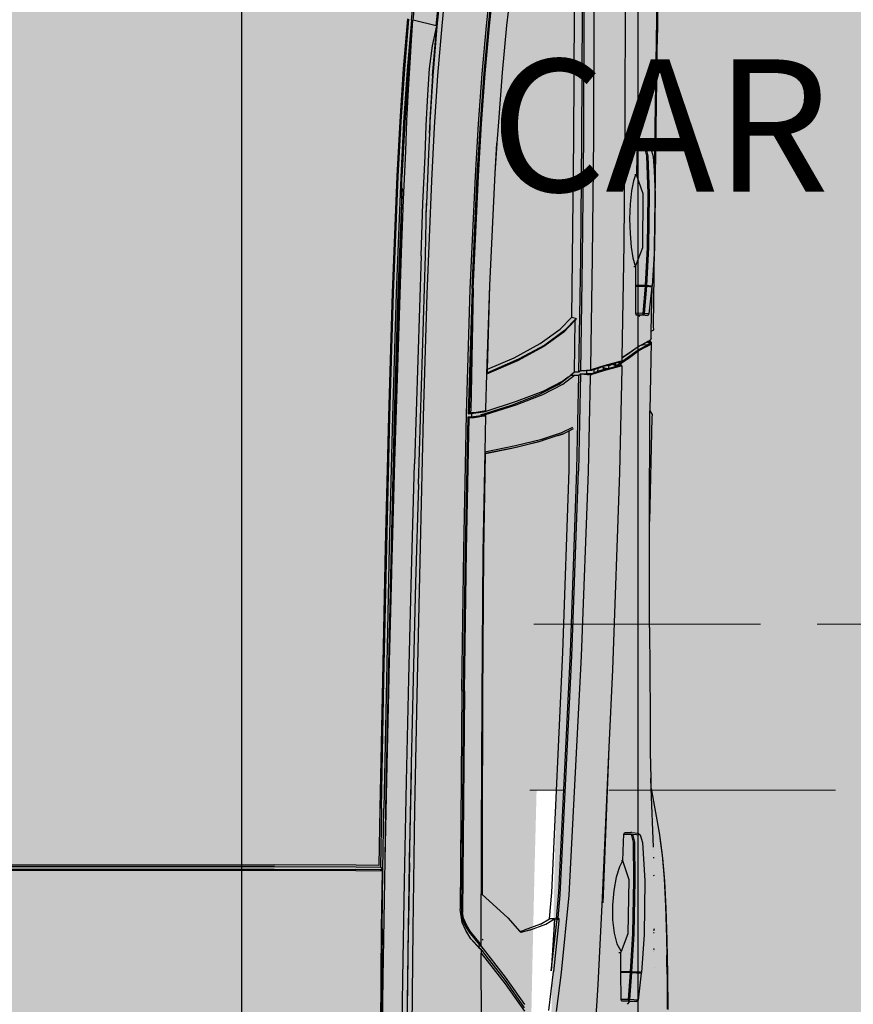
# Model space of a CAD drawing. Units: inches. Extents: x 1884 to 2398, y 474 to 1488.
# Tile 12 of 39: x 2231 to 2275, y 620 to 672. Entities that reach past the tile are written whole.
import ezdxf

# ---------------------------------------------------------------- set-up
doc = ezdxf.new("R2010")
doc.units = ezdxf.units.IN
doc.header["$MEASUREMENT"] = 0
doc.linetypes.add('ACAD_ISO02W100', pattern=[15, 12, -3])
doc.layers.get('0').update_dxf_attribs({"color": 250})
for name, color, linetype, lineweight in [('A-ANNO-DIMS', 2, 'Continuous', 18), ('A-FLOR-OVHD', 8, 'ACAD_ISO02W100', 18), ('C-VEHI', 8, 'Continuous', 18)]:
    doc.layers.add(name, color=color, linetype=linetype, lineweight=lineweight)
doc.layers.add('Edges', color=250, linetype='Continuous')
doc.layers.add('L-PVMT-PATT', color=9, linetype='Continuous', lineweight=13, true_color=0xc7c8ca)
doc.styles.get("Standard").update_dxf_attribs({"font": 'arial.ttf'})
doc.dimstyles.get("Standard").update_dxf_attribs({"dimtxt": 7, "dimasz": 0.18, "dimexe": 0.18, "dimexo": 0.0625, "dimgap": 0.09, "dimtad": 0, "dimtih": 1, "dimtoh": 1, "dimzin": 0, "dimdsep": 46, "dimlunit": 3, "dimtxsty": 'Standard', "dimcen": 0.09, "dimadec": 0, "dimazin": 0, "dimtfac": 1, "dimtofl": 0, "dimtmove": 0, "dimatfit": 3, "dimfxl": 1, "dimtolj": 1, "dimtzin": 0, "dimarcsym": 0})

# ---------------------------------------------------------------- blocks, each defined once
blk = doc.blocks.new('Nissan Qashqai pl')
at = {"layer": 'Edges'}
for p, q in [((10.4304, 12.8056), (10.4339, 12.8061)), ((10.4339, 12.8061), (10.4573, 12.8093)), ((10.4339, 12.8061), (10.4345, 12.8062)), ((10.4345, 12.8062), (10.4613, 12.8099)), ((10.4573, 12.8093), (10.4889, 12.8119)), ((10.4613, 12.8099), (10.4926, 12.8125)), ((10.4889, 12.8119), (10.526, 12.8138)), ((10.4926, 12.8125), (10.5294, 12.8143)), ((10.526, 12.8138), (10.569, 12.8151)), ((10.5294, 12.8143), (10.5719, 12.8156)), ((10.569, 12.8151), (10.5919, 12.8155)), ((10.5719, 12.8156), (10.6176, 12.8164)), ((10.5919, 12.8155), (10.6151, 12.8159)), ((10.5981, 12.8157), (10.5919, 12.8155)), ((10.6174, 12.816), (10.5981, 12.8157)), ((10.6151, 12.8159), (10.6644, 12.8162)), ((10.6176, 12.8164), (10.6651, 12.8167)), ((9.2517, 12.8031), (9.351, 12.803)), ((9.2517, 12.8031), (9.5372, 12.7983)), ((9.641, 12.7991), (9.351, 12.803)), ((9.5052, 12.7918), (9.5069, 12.7941)), ((9.5061, 12.7878), (9.5069, 12.7941)), ((9.5069, 12.7941), (9.5176, 12.7972)), ((9.5176, 12.7972), (9.5372, 12.7983)), ((9.5372, 12.7983), (9.5689, 12.7999)), ((9.5689, 12.7999), (9.641, 12.7991)), ((9.641, 12.7991), (9.6921, 12.7956)), ((9.7466, 12.7978), (9.641, 12.7991)), ((9.692, 12.7943), (9.6913, 12.7886)), ((9.6921, 12.7956), (9.692, 12.7943)), ((9.6922, 12.7943), (9.692, 12.7943)), ((9.6922, 12.7943), (9.6921, 12.7956)), ((9.7526, 12.7946), (9.6921, 12.7956)), ((9.6922, 12.7885), (9.693, 12.7955)), ((9.6922, 12.7885), (9.6922, 12.7943)), ((9.693, 12.7955), (9.7296, 12.7914)), ((9.7511, 12.7979), (9.7466, 12.7978)), ((9.7526, 12.7946), (9.7511, 12.7979)), ((9.7623, 12.7945), (9.7526, 12.7946)), ((9.7623, 12.7945), (9.7643, 12.7937)), ((9.7643, 12.7937), (9.7652, 12.7927)), ((9.7643, 12.7937), (9.7648, 12.7929)), ((9.7648, 12.7929), (9.7648, 12.7929)), ((9.7648, 12.7929), (9.7664, 12.7902)), ((9.7667, 12.7933), (9.7665, 12.7907)), ((9.7677, 12.7944), (9.7667, 12.7933)), ((9.7676, 12.7931), (9.7667, 12.7933)), ((9.7673, 12.7899), (9.7676, 12.7931)), ((9.769, 12.7926), (9.7676, 12.7931)), ((9.7677, 12.7944), (9.7677, 12.7944)), ((9.77, 12.7936), (9.7677, 12.7944)), ((9.7677, 12.7944), (9.8598, 12.7928)), ((9.7734, 12.7884), (9.77, 12.7936)), ((9.8598, 12.7928), (9.8614, 12.7937)), ((9.8614, 12.7937), (9.8647, 12.7956)), ((9.8647, 12.7956), (9.869, 12.7954)), ((9.869, 12.7954), (10.0085, 12.7922)), ((10.1513, 12.7924), (10.2677, 12.793)), ((10.2677, 12.793), (10.3189, 12.7931)), ((10.3189, 12.7931), (10.3537, 12.7939)), ((10.3537, 12.7939), (10.3832, 12.7945)), ((10.3679, 12.7944), (10.3537, 12.7939)), ((10.3679, 12.7944), (10.4275, 12.8051)), ((10.4468, 12.7976), (10.3679, 12.7944)), ((10.4275, 12.8051), (10.4304, 12.8056)), ((10.4503, 12.7976), (10.4502, 12.7976)), ((10.4603, 12.7976), (10.4613, 12.7978)), ((10.4838, 12.7977), (10.4852, 12.7982)), ((10.5565, 12.7985), (10.5591, 12.7977)), ((10.5615, 12.7978), (10.5617, 12.7985)), ((10.583, 12.7984), (10.5834, 12.798)), ((10.5836, 12.798), (10.5831, 12.7984)), ((10.5847, 12.798), (10.5841, 12.7984)), ((10.5873, 12.7981), (10.5873, 12.7981)), ((10.6087, 12.7983), (10.6087, 12.7984)), ((9.5037, 12.7806), (9.5045, 12.7814)), ((9.5052, 12.7918), (9.5044, 12.7856)), ((9.5044, 12.7856), (9.5045, 12.7814)), ((9.5045, 12.7814), (9.5045, 12.7759)), ((9.5168, 12.7904), (9.5061, 12.7878)), ((9.5061, 12.7856), (9.5167, 12.7883)), ((9.5063, 12.7755), (9.5061, 12.7856)), ((9.5167, 12.7883), (9.5679, 12.7899)), ((9.5679, 12.792), (9.5168, 12.7904)), ((9.5678, 12.7837), (9.5426, 12.7747)), ((9.64, 12.7831), (9.5678, 12.7837)), ((9.6401, 12.7914), (9.5679, 12.792)), ((9.5679, 12.7899), (9.64, 12.7892)), ((9.64, 12.7892), (9.6912, 12.7865)), ((9.6645, 12.7737), (9.64, 12.7831)), ((9.6913, 12.7886), (9.6401, 12.7914)), ((9.6912, 12.7811), (9.6911, 12.7796)), ((9.6911, 12.7796), (9.6911, 12.7732)), ((9.6913, 12.7886), (9.6912, 12.7865)), ((9.6912, 12.7865), (9.6912, 12.7811)), ((9.692, 12.7811), (9.6912, 12.7811)), ((9.692, 12.7811), (9.6921, 12.7864)), ((9.692, 12.7796), (9.692, 12.7811)), ((9.692, 12.7733), (9.692, 12.7796)), ((9.6922, 12.7885), (9.6921, 12.7864)), ((9.6921, 12.7864), (9.7288, 12.7832)), ((9.7288, 12.7854), (9.6922, 12.7885)), ((9.7288, 12.7832), (9.7287, 12.7734)), ((9.7296, 12.7914), (9.7288, 12.7854)), ((9.7306, 12.7834), (9.7288, 12.7854)), ((9.7288, 12.7854), (9.7288, 12.7832)), ((9.7288, 12.7832), (9.7306, 12.7834)), ((9.7296, 12.7914), (9.7314, 12.7895)), ((9.7305, 12.7738), (9.7306, 12.7834)), ((9.7305, 12.7738), (9.7313, 12.7798)), ((9.7306, 12.7834), (9.7314, 12.7895)), ((9.7314, 12.7895), (9.7313, 12.7798)), ((9.733, 12.7782), (9.7313, 12.7798)), ((9.7652, 12.7927), (9.7665, 12.7907)), ((9.7665, 12.7904), (9.7664, 12.7902)), ((9.7664, 12.7902), (9.7674, 12.7885)), ((9.7665, 12.7907), (9.7676, 12.7889)), ((9.7673, 12.7897), (9.7673, 12.7899)), ((9.7673, 12.7897), (9.7676, 12.7889)), ((9.7674, 12.7885), (9.7728, 12.7781)), ((9.7676, 12.7889), (9.7684, 12.7875)), ((9.7676, 12.7887), (9.7678, 12.7882)), ((9.7684, 12.7875), (9.7717, 12.781)), ((9.7712, 12.7892), (9.769, 12.7926)), ((9.7707, 12.7848), (9.7709, 12.7893)), ((9.7717, 12.781), (9.7707, 12.7848)), ((9.7709, 12.7893), (9.7712, 12.7892)), ((9.7724, 12.7874), (9.7712, 12.7892)), ((9.7717, 12.781), (9.7738, 12.7771)), ((9.7778, 12.777), (9.7724, 12.7874)), ((9.7788, 12.778), (9.7734, 12.7884)), ((9.8643, 12.7927), (9.8598, 12.7928)), ((10.0085, 12.7922), (9.8643, 12.7927)), ((10.0124, 12.7922), (10.0085, 12.7922)), ((10.1513, 12.7924), (10.0124, 12.7922)), ((10.4282, 12.7775), (10.4299, 12.7798)), ((10.4291, 12.77), (10.4299, 12.7798)), ((10.4299, 12.7798), (10.4406, 12.7829)), ((10.4406, 12.7829), (10.4919, 12.7858)), ((10.4919, 12.7858), (10.564, 12.7851)), ((10.564, 12.7851), (10.6151, 12.7813)), ((10.615, 12.7803), (10.6142, 12.7686)), ((10.6151, 12.7813), (10.615, 12.7803)), ((10.615, 12.7676), (10.6151, 12.7803)), ((10.6151, 12.7803), (10.615, 12.7803)), ((10.6151, 12.7803), (10.6151, 12.7813)), ((10.6151, 12.7685), (10.616, 12.7812)), ((10.616, 12.7812), (10.6526, 12.7768)), ((9.5045, 12.7759), (9.5063, 12.7755)), ((9.5063, 12.7755), (9.5168, 12.7751)), ((9.5168, 12.7751), (9.5423, 12.7746)), ((9.5423, 12.7746), (9.5422, 12.7736)), ((9.5422, 12.7736), (9.5422, 12.7725)), ((9.5422, 12.7736), (9.5424, 12.7735)), ((9.5426, 12.7747), (9.5423, 12.7746)), ((9.5426, 12.7747), (9.5424, 12.7735)), ((9.5424, 12.7735), (9.5503, 12.7706)), ((9.5503, 12.7706), (9.5641, 12.7681)), ((9.5641, 12.7681), (9.5818, 12.766)), ((9.6215, 12.766), (9.6395, 12.7676)), ((9.6395, 12.7676), (9.654, 12.7697)), ((9.654, 12.7697), (9.6633, 12.7726)), ((9.6633, 12.7726), (9.6645, 12.7737)), ((9.6655, 12.7733), (9.6645, 12.7737)), ((9.6655, 12.7733), (9.6911, 12.7732)), ((9.6655, 12.7713), (9.6655, 12.7733)), ((9.6911, 12.7732), (9.692, 12.7733)), ((9.692, 12.7733), (9.7287, 12.7734)), ((9.7287, 12.7734), (9.7305, 12.7738)), ((9.7728, 12.7781), (9.7832, 12.7637)), ((9.7738, 12.7771), (9.7842, 12.7627)), ((9.7883, 12.7626), (9.7778, 12.777)), ((9.7894, 12.7636), (9.7788, 12.778)), ((10.4263, 12.7665), (10.4274, 12.7674)), ((10.4282, 12.7775), (10.4274, 12.7679)), ((10.4274, 12.7679), (10.4274, 12.7674)), ((10.4274, 12.7674), (10.4275, 12.7586)), ((10.4398, 12.7724), (10.4291, 12.77)), ((10.4291, 12.7677), (10.4398, 12.7701)), ((10.4293, 12.7579), (10.4291, 12.7677)), ((10.4909, 12.773), (10.4398, 12.7724)), ((10.4398, 12.7701), (10.4909, 12.7708)), ((10.5631, 12.7715), (10.4909, 12.773)), ((10.4909, 12.7708), (10.563, 12.7692)), ((10.563, 12.7692), (10.6142, 12.7663)), ((10.6142, 12.7686), (10.5631, 12.7715)), ((10.6142, 12.7686), (10.6142, 12.7677)), ((10.6142, 12.7677), (10.615, 12.7676)), ((10.6142, 12.7677), (10.6142, 12.7663)), ((10.6151, 12.7676), (10.615, 12.7676)), ((10.6518, 12.7657), (10.6151, 12.7685)), ((10.6151, 12.7676), (10.6151, 12.7685)), ((10.6151, 12.7662), (10.6151, 12.7676)), ((10.6526, 12.7768), (10.6518, 12.7657)), ((10.6526, 12.7768), (10.6543, 12.7749)), ((10.6537, 12.7658), (10.6543, 12.7749)), ((10.6543, 12.7749), (10.6543, 12.7656)), ((9.2886, 12.7594), (9.4673, 12.7589)), ((9.4673, 12.7589), (9.6358, 12.7575)), ((9.5818, 12.766), (9.6016, 12.7651)), ((9.6016, 12.7651), (9.6215, 12.766)), ((9.6358, 12.7575), (9.7887, 12.7552)), ((9.7832, 12.7637), (9.7887, 12.7552)), ((9.7842, 12.7627), (9.7891, 12.7552)), ((9.7933, 12.7549), (9.7883, 12.7626)), ((9.7887, 12.7552), (9.7891, 12.7552)), ((9.7891, 12.7552), (9.79, 12.7552)), ((9.7965, 12.7526), (9.7894, 12.7636)), ((9.79, 12.7552), (9.7931, 12.7552)), ((9.7931, 12.7552), (9.7934, 12.7535)), ((9.7931, 12.7552), (9.7933, 12.7549)), ((9.7933, 12.7549), (9.7941, 12.7541)), ((9.7934, 12.7535), (9.7938, 12.7538)), ((9.7934, 12.7535), (9.7937, 12.7524)), ((9.7941, 12.7541), (9.7943, 12.7535)), ((9.7955, 12.7516), (9.7943, 12.7535)), ((9.7943, 12.7535), (9.7964, 12.7453)), ((9.7983, 12.7541), (9.7965, 12.7526)), ((9.7977, 12.7535), (9.7967, 12.7526)), ((9.7982, 12.754), (9.7977, 12.7535)), ((9.7983, 12.7541), (9.7982, 12.754)), ((9.7986, 12.7526), (9.7982, 12.754)), ((9.7986, 12.7544), (9.7983, 12.7541)), ((9.7993, 12.755), (9.7986, 12.7544)), ((9.7999, 12.7522), (9.7993, 12.755)), ((9.7993, 12.755), (9.8024, 12.7549)), ((9.8024, 12.7549), (9.9426, 12.7518)), ((10.4293, 12.7579), (10.4275, 12.7586)), ((10.4398, 12.7573), (10.4293, 12.7579)), ((10.4653, 12.7564), (10.4398, 12.7573)), ((10.4653, 12.7561), (10.4652, 12.7545)), ((10.4908, 12.7648), (10.4653, 12.7564)), ((10.4653, 12.7564), (10.4653, 12.7561)), ((10.4653, 12.7564), (10.4653, 12.7564)), ((10.4653, 12.7564), (10.4653, 12.7561)), ((10.4653, 12.7561), (10.4653, 12.7561)), ((10.4653, 12.7561), (10.4732, 12.7517)), ((10.563, 12.7633), (10.4908, 12.7648)), ((10.5867, 12.7545), (10.563, 12.7633)), ((10.5769, 12.7484), (10.5863, 12.7537)), ((10.5863, 12.7537), (10.5867, 12.7545)), ((10.5885, 12.7538), (10.5867, 12.7545)), ((10.5885, 12.751), (10.5885, 12.7538)), ((10.6141, 12.7537), (10.5885, 12.7538)), ((10.6142, 12.766), (10.6141, 12.7537)), ((10.6141, 12.7537), (10.615, 12.7537)), ((10.6142, 12.7663), (10.6142, 12.766)), ((10.615, 12.7537), (10.6151, 12.7659)), ((10.6517, 12.754), (10.615, 12.7537)), ((10.6151, 12.7662), (10.6518, 12.7634)), ((10.6151, 12.7659), (10.6151, 12.7662)), ((10.6518, 12.7634), (10.6517, 12.754)), ((10.6535, 12.7546), (10.6517, 12.754)), ((10.6536, 12.7639), (10.6518, 12.7657)), ((10.6518, 12.7657), (10.6518, 12.7634)), ((10.6518, 12.7634), (10.6536, 12.7639)), ((10.6543, 12.7656), (10.6535, 12.7546)), ((10.6535, 12.7546), (10.6536, 12.7639)), ((10.6536, 12.7639), (10.6537, 12.7658)), ((10.6537, 12.7658), (10.6543, 12.7656)), ((10.6578, 12.7628), (10.6543, 12.7656)), ((9.7937, 12.7524), (9.7992, 12.7308)), ((9.7963, 12.7523), (9.7955, 12.7516)), ((9.7963, 12.7523), (9.7963, 12.7524)), ((9.7964, 12.7524), (9.7963, 12.7523)), ((9.7992, 12.7476), (9.7963, 12.7523)), ((9.7967, 12.7526), (9.7964, 12.7524)), ((9.7964, 12.7525), (9.7964, 12.7524)), ((9.7964, 12.7524), (9.7996, 12.7475)), ((9.7964, 12.7453), (9.7992, 12.7476)), ((9.7964, 12.7453), (9.7973, 12.7418)), ((9.7965, 12.7526), (9.7967, 12.7526)), ((9.7967, 12.7526), (9.7986, 12.7526)), ((9.7977, 12.7431), (9.7973, 12.7418)), ((9.7973, 12.7418), (9.7977, 12.7409)), ((9.7973, 12.7418), (9.7977, 12.7399)), ((9.7977, 12.7444), (9.7985, 12.7451)), ((9.7985, 12.7451), (9.7977, 12.7431)), ((9.7977, 12.7431), (9.7977, 12.7444)), ((9.7977, 12.7399), (9.7977, 12.7409)), ((9.7977, 12.7409), (9.7987, 12.7388)), ((9.7977, 12.7399), (9.7978, 12.7397)), ((9.7989, 12.7461), (9.7985, 12.7451)), ((9.7988, 12.7516), (9.7986, 12.7526)), ((9.7998, 12.7477), (9.7988, 12.7516)), ((9.7998, 12.7466), (9.7989, 12.7461)), ((9.7998, 12.7466), (9.7992, 12.7476)), ((9.7996, 12.7475), (9.7998, 12.7477)), ((9.8002, 12.7461), (9.7996, 12.7475)), ((9.8001, 12.7468), (9.7996, 12.7475)), ((9.8001, 12.7468), (9.7998, 12.7477)), ((9.8003, 12.7458), (9.7998, 12.7466)), ((9.8054, 12.7307), (9.7999, 12.7522)), ((9.8002, 12.7461), (9.8001, 12.7468)), ((9.8003, 12.7458), (9.8002, 12.7461)), ((9.8027, 12.7364), (9.8003, 12.7458)), ((9.9426, 12.7518), (10.2081, 12.7424)), ((10.2081, 12.7424), (10.312, 12.7377)), ((10.4732, 12.7517), (10.4871, 12.7474)), ((10.4871, 12.7474), (10.5048, 12.744)), ((10.5048, 12.744), (10.5246, 12.7423)), ((10.5246, 12.7423), (10.5445, 12.7425)), ((10.5445, 12.7425), (10.5625, 12.7446)), ((10.5625, 12.7446), (10.5769, 12.7484)), ((9.7987, 12.7388), (9.7978, 12.7397)), ((9.7978, 12.7397), (9.7987, 12.7362)), ((9.7987, 12.7388), (9.7992, 12.7377)), ((9.7987, 12.7362), (9.7992, 12.7377)), ((9.7987, 12.7362), (9.8002, 12.7301)), ((9.7992, 12.7377), (9.8027, 12.7364)), ((9.7992, 12.7308), (9.8044, 12.7151)), ((9.8002, 12.7301), (9.8008, 12.7285)), ((9.8008, 12.7285), (9.8014, 12.7303)), ((9.8008, 12.7285), (9.8014, 12.7265)), ((9.8014, 12.7303), (9.8031, 12.7349)), ((9.8043, 12.7303), (9.8014, 12.7303)), ((9.8031, 12.7349), (9.8027, 12.7364)), ((9.8043, 12.7303), (9.8031, 12.7349)), ((9.8044, 12.73), (9.8043, 12.7303)), ((9.8067, 12.7229), (9.8044, 12.73)), ((9.8106, 12.715), (9.8054, 12.7307)), ((10.312, 12.7377), (10.5214, 12.7293)), ((10.312, 12.7377), (10.5147, 12.7285)), ((10.5147, 12.7285), (10.6318, 12.7228)), ((9.4919, 12.7173), (9.3194, 12.7179)), ((9.6538, 12.7157), (9.4919, 12.7173)), ((9.802, 12.7133), (9.6538, 12.7157)), ((9.8014, 12.7265), (9.803, 12.723)), ((9.8014, 12.7265), (9.8026, 12.723)), ((9.803, 12.723), (9.8026, 12.723)), ((9.8026, 12.723), (9.8046, 12.7171)), ((9.8067, 12.7229), (9.803, 12.723)), ((9.8044, 12.7151), (9.8051, 12.7132)), ((9.8046, 12.7171), (9.8086, 12.7171)), ((9.8046, 12.7171), (9.8055, 12.7143)), ((9.8055, 12.7143), (9.8058, 12.7073)), ((9.8086, 12.7171), (9.8067, 12.7229)), ((9.8096, 12.7142), (9.8086, 12.7171)), ((9.8098, 12.7073), (9.8096, 12.7142)), ((9.8112, 12.7131), (9.8106, 12.715)), ((10.6318, 12.7228), (10.6955, 12.7184)), ((9.3198, 12.7039), (9.4922, 12.7033)), ((9.4936, 12.7013), (9.3225, 12.7021)), ((9.4922, 12.7033), (9.654, 12.7018)), ((9.6552, 12.6997), (9.4936, 12.7013)), ((9.654, 12.7018), (9.8061, 12.6994)), ((9.8051, 12.7132), (9.802, 12.7133)), ((9.8061, 12.6994), (9.8051, 12.7132)), ((9.8058, 12.7073), (9.8098, 12.7073)), ((9.8058, 12.7073), (9.8061, 12.6994)), ((9.8101, 12.6993), (9.8098, 12.7073)), ((9.8101, 12.6993), (9.8112, 12.7131)), ((9.8143, 12.713), (9.8112, 12.7131)), ((9.9414, 12.71), (9.8143, 12.713)), ((10.19, 12.7008), (9.9414, 12.71)), ((10.5113, 12.6839), (10.19, 12.7008)), ((9.4936, 12.6904), (9.3225, 12.6911)), ((9.6552, 12.6888), (9.4936, 12.6904)), ((9.8078, 12.6971), (9.6552, 12.6997)), ((9.7337, 12.6875), (9.6552, 12.6888)), ((9.7337, 12.6875), (9.7357, 12.6935)), ((9.7499, 12.6721), (9.7337, 12.6875)), ((9.7357, 12.6935), (9.7378, 12.6924)), ((9.7357, 12.6935), (9.7519, 12.678)), ((9.7378, 12.6924), (9.754, 12.677)), ((9.8078, 12.6913), (9.7378, 12.6924)), ((9.8061, 12.6994), (9.8078, 12.6971)), ((9.8078, 12.6971), (9.8078, 12.6913)), ((9.8078, 12.6913), (9.8119, 12.6862)), ((9.8119, 12.697), (9.8101, 12.6993)), ((9.8101, 12.6993), (9.9411, 12.6966)), ((9.9393, 12.6944), (9.8119, 12.697)), ((9.8119, 12.6912), (9.8119, 12.697)), ((9.8241, 12.6756), (9.8119, 12.6912)), ((9.8119, 12.6862), (9.8119, 12.6912)), ((9.8891, 12.6741), (9.8818, 12.6891)), ((9.8867, 12.6842), (9.8838, 12.6901)), ((10.1849, 12.6857), (9.9393, 12.6944)), ((10.1894, 12.6879), (9.9411, 12.6966)), ((10.5109, 12.6721), (10.1894, 12.6879)), ((9.7519, 12.678), (9.7713, 12.6512)), ((9.754, 12.677), (9.7733, 12.6502)), ((9.8147, 12.6826), (9.8119, 12.6862)), ((9.8147, 12.6826), (9.8147, 12.6826)), ((9.8147, 12.6826), (9.8201, 12.6756)), ((9.8241, 12.6706), (9.8147, 12.6826)), ((9.8201, 12.6756), (9.8338, 12.6486)), ((9.8378, 12.6485), (9.8241, 12.6756)), ((9.9393, 12.684), (9.8867, 12.6842)), ((9.8911, 12.675), (9.8867, 12.6842)), ((9.8978, 12.6472), (9.8891, 12.6741)), ((9.8911, 12.6749), (9.8911, 12.675)), ((9.8931, 12.6691), (9.8911, 12.6749)), ((9.8911, 12.6749), (9.8998, 12.6481)), ((10.1849, 12.6754), (9.9393, 12.684)), ((10.5079, 12.6703), (10.1849, 12.6857)), ((10.5079, 12.6607), (10.1849, 12.6754)), ((10.6152, 12.674), (10.5113, 12.6839)), ((10.6678, 12.6672), (10.6152, 12.674)), ((9.7692, 12.6453), (9.7499, 12.6721)), ((9.8378, 12.6435), (9.8241, 12.6706)), ((9.8931, 12.669), (9.8931, 12.6691)), ((9.8931, 12.669), (9.9018, 12.6421)), ((10.543, 12.6671), (10.5079, 12.6703)), ((10.543, 12.6576), (10.5079, 12.6607)), ((10.5417, 12.6693), (10.5109, 12.6721)), ((10.5417, 12.6693), (10.5427, 12.6702)), ((10.5417, 12.6693), (10.543, 12.6671)), ((10.5436, 12.6687), (10.5427, 12.6702)), ((10.5427, 12.6702), (10.5458, 12.67)), ((10.544, 12.6678), (10.543, 12.6671)), ((10.543, 12.6646), (10.543, 12.6671)), ((10.543, 12.6646), (10.543, 12.6576)), ((10.5439, 12.6646), (10.543, 12.6646)), ((10.5502, 12.6526), (10.543, 12.6646)), ((10.544, 12.6678), (10.5436, 12.6687)), ((10.5439, 12.6646), (10.613, 12.6601)), ((10.547, 12.6674), (10.544, 12.6678)), ((10.5458, 12.67), (10.6144, 12.6629)), ((10.613, 12.6601), (10.547, 12.6674)), ((10.6664, 12.6566), (10.6144, 12.6629)), ((9.7713, 12.6512), (9.7905, 12.6158)), ((9.7733, 12.6502), (9.7925, 12.6148)), ((9.8338, 12.6486), (9.8475, 12.613)), ((9.8516, 12.6129), (9.8378, 12.6485)), ((9.9066, 12.6119), (9.8978, 12.6472)), ((9.9086, 12.6129), (9.8998, 12.6481)), ((10.5502, 12.6456), (10.543, 12.6576)), ((10.5584, 12.6306), (10.5502, 12.6526)), ((9.7885, 12.6099), (9.7692, 12.6453)), ((9.8516, 12.6079), (9.8378, 12.6435)), ((9.9018, 12.6421), (9.9106, 12.6068)), ((10.5502, 12.6456), (10.5584, 12.6236)), ((10.5584, 12.6306), (10.5617, 12.619)), ((10.56, 12.6176), (10.5584, 12.6236)), ((10.6583, 12.6245), (10.6215, 12.5986)), ((10.6627, 12.6241), (10.6261, 12.5984)), ((10.6306, 12.5982), (10.6671, 12.6238)), ((9.8039, 12.5741), (9.7885, 12.6099)), ((9.7905, 12.6158), (9.8087, 12.574)), ((9.7925, 12.6148), (9.8107, 12.573)), ((9.8475, 12.613), (9.8611, 12.5708)), ((9.8652, 12.5704), (9.8516, 12.6129)), ((9.8652, 12.5654), (9.8516, 12.6079)), ((9.9149, 12.5705), (9.9066, 12.6119)), ((9.9169, 12.5714), (9.9086, 12.6129)), ((10.5419, 12.6018), (10.56, 12.6176)), ((10.56, 12.6176), (10.5617, 12.619)), ((9.2814, 12.6065), (9.3416, 12.5999)), ((9.3416, 12.5999), (9.4048, 12.5941)), ((9.9106, 12.6068), (9.9177, 12.5714)), ((10.51, 12.5666), (10.5419, 12.6018)), ((10.6215, 12.5986), (10.5796, 12.5655)), ((10.5892, 12.5659), (10.6306, 12.5982)), ((10.6261, 12.5984), (10.593, 12.5726)), ((9.3418, 12.5771), (9.2803, 12.5836)), ((9.3419, 12.5756), (9.2804, 12.5821)), ((9.4048, 12.5941), (9.471, 12.5888)), ((9.471, 12.5888), (9.4997, 12.5869)), ((9.5404, 12.5844), (9.4997, 12.5869)), ((9.4997, 12.5869), (9.5403, 12.5842)), ((9.5403, 12.5842), (9.6913, 12.5767)), ((9.6912, 12.5774), (9.5404, 12.5844)), ((9.3418, 12.5729), (9.2801, 12.5794)), ((9.4062, 12.5713), (9.3418, 12.5771)), ((9.4064, 12.5671), (9.3418, 12.5729)), ((9.4063, 12.5699), (9.3419, 12.5756)), ((9.4735, 12.5663), (9.4062, 12.5713)), ((9.4736, 12.5648), (9.4063, 12.5699)), ((9.8039, 12.5741), (9.6912, 12.5774)), ((9.6913, 12.5767), (9.8099, 12.573)), ((9.8087, 12.574), (9.8039, 12.5741)), ((9.8099, 12.573), (9.8087, 12.574)), ((9.8099, 12.573), (9.8107, 12.573)), ((9.8107, 12.573), (9.8573, 12.5716)), ((9.8573, 12.5716), (9.8603, 12.5715)), ((9.8603, 12.5715), (9.8605, 12.5696)), ((9.8611, 12.5708), (9.8603, 12.5715)), ((9.8605, 12.5696), (9.8626, 12.5564)), ((9.8612, 12.5707), (9.8611, 12.5708)), ((9.8612, 12.5707), (9.8615, 12.5688)), ((9.8615, 12.5688), (9.8635, 12.5556)), ((9.8652, 12.5706), (9.8664, 12.5714)), ((9.8652, 12.5706), (9.8665, 12.5695)), ((9.8652, 12.5704), (9.8652, 12.5706)), ((9.8652, 12.5704), (9.8652, 12.5704)), ((9.8652, 12.5704), (9.8652, 12.5654)), ((9.8655, 12.5687), (9.8652, 12.5704)), ((9.8675, 12.5555), (9.8655, 12.5687)), ((9.8665, 12.5695), (9.8664, 12.5714)), ((9.8664, 12.5714), (9.9149, 12.5705)), ((9.8686, 12.5562), (9.8665, 12.5695)), ((9.9149, 12.5705), (10.0505, 12.5681)), ((9.9177, 12.5714), (9.9169, 12.5714)), ((10.0501, 12.5695), (9.9177, 12.5714)), ((10.2453, 12.568), (10.0501, 12.5695)), ((10.0505, 12.5681), (10.2453, 12.5664)), ((10.4292, 12.5674), (10.2453, 12.568)), ((10.5719, 12.5682), (10.5709, 12.5675)), ((10.593, 12.5726), (10.584, 12.5655)), ((9.4739, 12.5621), (9.4064, 12.5671)), ((9.5437, 12.5619), (9.4735, 12.5663)), ((9.5438, 12.5605), (9.4736, 12.5648)), ((9.5443, 12.5579), (9.4739, 12.5621)), ((9.6953, 12.5549), (9.5437, 12.5619)), ((9.6954, 12.5535), (9.5438, 12.5605)), ((9.696, 12.551), (9.5443, 12.5579)), ((9.6953, 12.5549), (9.8598, 12.5517)), ((9.6953, 12.5549), (9.863, 12.5497)), ((9.8626, 12.5564), (9.8627, 12.5532)), ((9.8635, 12.5556), (9.8637, 12.5532)), ((9.8677, 12.5531), (9.8675, 12.5555)), ((9.8689, 12.5515), (9.8686, 12.5562)), ((10.2453, 12.5664), (10.4289, 12.5658)), ((10.4289, 12.5658), (10.5092, 12.5658)), ((10.5099, 12.5674), (10.4292, 12.5674)), ((10.5099, 12.5674), (10.5092, 12.5658)), ((10.5092, 12.5658), (10.5094, 12.5658)), ((10.5094, 12.5658), (10.51, 12.5666)), ((10.5783, 12.5659), (10.5094, 12.5658)), ((10.51, 12.5666), (10.5099, 12.5674)), ((10.5764, 12.5642), (10.5598, 12.5507)), ((10.5776, 12.5633), (10.5612, 12.5498)), ((10.5834, 12.5641), (10.57, 12.5517)), ((10.57, 12.5517), (10.5821, 12.5633)), ((10.5709, 12.5675), (10.5705, 12.5671)), ((10.5783, 12.5659), (10.5764, 12.5642)), ((10.5776, 12.5633), (10.5783, 12.5659)), ((10.5796, 12.5655), (10.5776, 12.5633)), ((10.5796, 12.5655), (10.5783, 12.5659)), ((10.5796, 12.562), (10.5796, 12.5655)), ((10.5838, 12.5653), (10.5821, 12.5633)), ((10.584, 12.5647), (10.5834, 12.5641)), ((10.584, 12.5655), (10.5838, 12.5653)), ((10.584, 12.5655), (10.5841, 12.5655)), ((10.584, 12.5654), (10.584, 12.5655)), ((10.5847, 12.5655), (10.584, 12.5647)), ((10.584, 12.5647), (10.584, 12.5654)), ((10.5851, 12.5659), (10.5841, 12.5655)), ((10.5841, 12.5655), (10.5847, 12.5655)), ((10.5851, 12.5659), (10.5847, 12.5655)), ((10.5851, 12.5659), (10.5892, 12.5659)), ((10.6988, 12.5662), (10.5892, 12.5659)), ((9.6954, 12.5535), (9.8641, 12.5483)), ((9.8644, 12.5459), (9.696, 12.551)), ((9.8629, 12.5516), (9.8598, 12.5517)), ((9.8637, 12.5532), (9.8627, 12.5532)), ((9.8627, 12.5532), (9.8629, 12.5516)), ((9.8629, 12.5516), (9.863, 12.5497)), ((9.8641, 12.5483), (9.863, 12.5497)), ((9.8643, 12.5532), (9.8637, 12.5532)), ((9.8637, 12.5532), (9.8638, 12.5508)), ((9.8638, 12.5508), (9.8641, 12.5483)), ((9.8677, 12.5531), (9.8643, 12.5532)), ((10.0472, 12.5423), (9.8644, 12.5459)), ((9.8678, 12.5507), (9.8677, 12.5531)), ((9.8681, 12.5482), (9.8678, 12.5507)), ((9.8681, 12.5482), (9.869, 12.5496)), ((10.0476, 12.5445), (9.8681, 12.5482)), ((9.869, 12.5496), (9.8689, 12.5515)), ((10.0477, 12.5459), (9.869, 12.5496)), ((10.2357, 12.5398), (10.0472, 12.5423)), ((10.2367, 12.5419), (10.0476, 12.5445)), ((10.2369, 12.5433), (10.0477, 12.5459)), ((10.2367, 12.5419), (10.5351, 12.5392)), ((10.2369, 12.5433), (10.5348, 12.5406)), ((10.5422, 12.542), (10.5348, 12.5406)), ((10.5522, 12.5465), (10.5422, 12.542)), ((10.5495, 12.5438), (10.5424, 12.5406)), ((10.5463, 12.541), (10.5551, 12.5457)), ((10.5589, 12.5451), (10.5479, 12.54)), ((10.5546, 12.546), (10.5495, 12.5438)), ((10.5598, 12.5507), (10.5522, 12.5465)), ((10.5583, 12.5481), (10.5546, 12.546)), ((10.5551, 12.5457), (10.5583, 12.5481)), ((10.5612, 12.5498), (10.5583, 12.5481)), ((10.57, 12.5517), (10.5589, 12.5451)), ((10.2357, 12.5398), (10.53, 12.5373)), ((10.4153, 12.5384), (10.4176, 12.5384)), ((10.4176, 12.5384), (10.4181, 12.5384)), ((10.4181, 12.5384), (10.4552, 12.538)), ((10.4181, 12.5384), (10.4181, 12.5384)), ((10.4778, 12.5378), (10.53, 12.5373)), ((10.5301, 12.5373), (10.53, 12.5373)), ((10.5335, 12.5378), (10.5301, 12.5373)), ((10.5419, 12.5391), (10.5335, 12.5378)), ((10.5418, 12.5405), (10.5351, 12.5392)), ((10.5424, 12.5406), (10.5418, 12.5405)), ((10.5419, 12.5391), (10.5463, 12.541)), ((10.5479, 12.54), (10.5419, 12.5391)), ((9.2783, 12.5191), (9.3422, 12.5126)), ((9.3427, 12.5066), (9.2789, 12.5131)), ((9.3418, 12.5051), (9.2819, 12.5112)), ((9.3418, 12.5051), (9.3346, 12.4741)), ((9.342, 12.5059), (9.3418, 12.5051)), ((9.3687, 12.5), (9.342, 12.5059)), ((9.4087, 12.5003), (9.342, 12.5059)), ((9.3422, 12.5126), (9.4088, 12.507)), ((9.4093, 12.5011), (9.3427, 12.5066)), ((9.4088, 12.507), (9.4782, 12.5024)), ((9.4782, 12.5024), (9.5503, 12.4987)), ((9.3992, 12.496), (9.3687, 12.5)), ((9.4347, 12.494), (9.3992, 12.496)), ((9.4087, 12.5003), (9.4688, 12.4968)), ((9.4785, 12.4965), (9.4093, 12.5011)), ((9.4761, 12.4919), (9.4347, 12.494)), ((9.4688, 12.4968), (9.4789, 12.4964)), ((9.5168, 12.4903), (9.4761, 12.4919)), ((9.4789, 12.4964), (9.4785, 12.4965)), ((9.4862, 12.4961), (9.4785, 12.4965)), ((9.4789, 12.4964), (9.4862, 12.4961)), ((9.4862, 12.4961), (9.514, 12.4949)), ((9.514, 12.4949), (9.5811, 12.492)), ((9.5812, 12.4874), (9.5168, 12.4903)), ((9.5503, 12.4987), (9.7029, 12.4926)), ((9.651, 12.4906), (9.5811, 12.492)), ((9.5811, 12.492), (9.594, 12.4914)), ((9.9583, 12.4812), (9.651, 12.4906)), ((9.7029, 12.4926), (9.8673, 12.4878)), ((9.3346, 12.4718), (9.2704, 12.4783)), ((9.3346, 12.4741), (9.2724, 12.4804)), ((9.6514, 12.4849), (9.5812, 12.4874)), ((9.6514, 12.4849), (9.9312, 12.4761)), ((9.8673, 12.4878), (10.0423, 12.4835)), ((10.0776, 12.4719), (9.9312, 12.4761)), ((9.9583, 12.4812), (10.091, 12.4775)), ((10.0423, 12.4835), (10.2211, 12.4795)), ((10.091, 12.4775), (10.2202, 12.4743)), ((10.2211, 12.4795), (10.3955, 12.4762)), ((10.3955, 12.4762), (10.5572, 12.4737)), ((9.3326, 12.4666), (9.4, 12.4609)), ((9.4004, 12.4629), (9.333, 12.4685)), ((9.3346, 12.4741), (9.3344, 12.4733)), ((9.3344, 12.4733), (9.4017, 12.4677)), ((9.3344, 12.4733), (9.3611, 12.4715)), ((9.3346, 12.4718), (9.4018, 12.4661)), ((9.3611, 12.4715), (9.3918, 12.4695)), ((9.3918, 12.4695), (9.4276, 12.4674)), ((9.4709, 12.4581), (9.4004, 12.4629)), ((9.4017, 12.4677), (9.472, 12.463)), ((9.4018, 12.4661), (9.472, 12.4614)), ((9.4276, 12.4674), (9.4694, 12.4654)), ((9.4694, 12.4654), (9.5105, 12.4637)), ((9.472, 12.463), (9.5454, 12.4591)), ((9.5105, 12.4637), (9.5755, 12.4608)), ((10.2201, 12.4683), (10.0776, 12.4719)), ((10.3586, 12.4651), (10.2201, 12.4683)), ((10.2202, 12.4743), (10.2203, 12.4743)), ((10.2203, 12.4743), (10.3353, 12.4717)), ((10.3353, 12.4717), (10.4477, 12.4694)), ((10.3353, 12.4717), (10.346, 12.4714)), ((10.346, 12.4714), (10.4477, 12.4694)), ((10.4931, 12.4624), (10.3586, 12.4651)), ((10.4477, 12.4694), (10.4538, 12.4693)), ((10.4538, 12.4693), (10.4681, 12.469)), ((10.4676, 12.4691), (10.4538, 12.4693)), ((10.5566, 12.4677), (10.4676, 12.4691)), ((10.4676, 12.4691), (10.546, 12.4677)), ((10.4681, 12.469), (10.5866, 12.467)), ((10.6237, 12.4603), (10.4931, 12.4624)), ((10.546, 12.4677), (10.546, 12.4678)), ((10.546, 12.4677), (10.5576, 12.4675)), ((10.7, 12.4662), (10.5566, 12.4677)), ((10.5572, 12.4737), (10.7004, 12.4722)), ((10.5576, 12.4675), (10.6649, 12.4659)), ((10.5866, 12.467), (10.6649, 12.4659)), ((9.4, 12.4609), (9.4706, 12.4561)), ((9.4706, 12.4561), (9.5443, 12.4522)), ((9.5446, 12.4542), (9.4709, 12.4581)), ((9.472, 12.4614), (9.5454, 12.4576)), ((9.5443, 12.4522), (9.701, 12.4459)), ((9.7011, 12.4478), (9.5446, 12.4542)), ((9.5454, 12.4591), (9.5454, 12.4593)), ((9.5695, 12.4589), (9.5454, 12.4591)), ((9.5454, 12.4576), (9.7014, 12.4513)), ((9.5609, 12.4593), (9.5695, 12.4589)), ((9.5786, 12.4588), (9.5695, 12.4589)), ((9.5695, 12.4589), (9.7014, 12.4536)), ((9.5755, 12.4608), (9.6472, 12.4581)), ((9.6206, 12.4581), (9.5786, 12.4588)), ((9.6714, 12.4567), (9.6206, 12.4581)), ((9.6414, 12.458), (9.6407, 12.458)), ((9.6472, 12.4581), (9.9278, 12.4492)), ((9.6549, 12.4576), (9.6558, 12.4574)), ((9.6825, 12.4564), (9.6714, 12.4567)), ((9.6825, 12.4564), (9.6829, 12.4563)), ((9.6943, 12.456), (9.6825, 12.4564)), ((9.6943, 12.4558), (9.6943, 12.456)), ((9.6951, 12.456), (9.6943, 12.456)), ((9.6951, 12.4558), (9.6951, 12.456)), ((9.8565, 12.451), (9.6951, 12.456)), ((9.7014, 12.4536), (9.8673, 12.4488)), ((9.7014, 12.4513), (9.8673, 12.4464)), ((9.9794, 12.4475), (9.8565, 12.451)), ((9.8673, 12.4488), (10.0429, 12.4444)), ((9.9278, 12.4492), (10.0747, 12.445)), ((10.7502, 12.4586), (10.6237, 12.4603)), ((9.701, 12.4459), (9.8673, 12.441)), ((9.8673, 12.443), (9.7011, 12.4478)), ((9.8673, 12.4464), (10.0429, 12.4421)), ((10.043, 12.4387), (9.8673, 12.443)), ((9.8673, 12.441), (10.0431, 12.4367)), ((10.0998, 12.4443), (9.9794, 12.4475)), ((10.0429, 12.4444), (10.2216, 12.4404)), ((10.0429, 12.4421), (10.2215, 12.4381)), ((10.2218, 12.4347), (10.043, 12.4387)), ((10.0431, 12.4367), (10.2218, 12.4327)), ((10.0747, 12.445), (10.078, 12.4449)), ((10.078, 12.4449), (10.2146, 12.4414)), ((10.2146, 12.4414), (10.0998, 12.4443)), ((10.2146, 12.4414), (10.2175, 12.4413)), ((10.2175, 12.4413), (10.3564, 12.4382)), ((10.2215, 12.4381), (10.3945, 12.4348)), ((10.2216, 12.4404), (10.3947, 12.4371)), ((10.3564, 12.4382), (10.4638, 12.436)), ((10.3947, 12.4371), (10.4638, 12.436)), ((10.4638, 12.436), (10.4914, 12.4355)), ((10.4914, 12.4355), (10.6223, 12.4333)), ((10.3947, 12.4314), (10.2218, 12.4347)), ((10.2218, 12.4327), (10.3947, 12.4294)), ((10.4773, 12.4335), (10.3945, 12.4348)), ((10.3947, 12.4314), (10.4735, 12.4301)), ((10.3947, 12.4294), (10.4715, 12.4282)), ((10.4715, 12.4282), (10.4711, 12.3973)), ((10.4731, 12.3973), (10.4735, 12.4301)), ((10.4735, 12.4301), (10.4773, 12.4335)), ((10.4773, 12.4296), (10.4769, 12.3968)), ((10.4773, 12.4335), (10.4773, 12.4296)), ((10.4785, 12.433), (10.4773, 12.4335)), ((10.5561, 12.4323), (10.4773, 12.4335)), ((10.4781, 12.3972), (10.4785, 12.433)), ((10.5563, 12.4318), (10.4785, 12.433)), ((10.5561, 12.4323), (10.6996, 12.4308)), ((10.6999, 12.4304), (10.5563, 12.4318)), ((10.6223, 12.4333), (10.7493, 12.4316)), ((10.4711, 12.3973), (10.4706, 12.2875)), ((10.4726, 12.2875), (10.4731, 12.3973)), ((10.4764, 12.2872), (10.4769, 12.3968)), ((10.4776, 12.2874), (10.4781, 12.3972)), ((10.4706, 11.5566), (10.4706, 12.2875)), ((10.4726, 11.5567), (10.4726, 12.2875)), ((10.4764, 11.5569), (10.4764, 12.2872)), ((10.4776, 11.5567), (10.4776, 12.2874))]:
    blk.add_line(p, q, dxfattribs=at)
blk = doc.blocks.new('car')
blk.add_blockref('Nissan Qashqai pl', (-9.7433, -11.9151))
blk = doc.blocks.new('carr')
blk.add_blockref('car', (0.5124, -0.007))
blk = doc.blocks.new('*D23')
at = {"layer": 'A-ANNO-DIMS', "color": 0, "lineweight": -2, "transparency": 16777216}
for p, q in [((2272.304, 752.812), (2298.291, 752.812)), ((2298.111, 752.632), (2298.111, 670.29)), ((2298.111, 580.529), (2298.111, 662.871)), ((2272.304, 580.349), (2298.291, 580.349))]:
    blk.add_line(p, q, dxfattribs=at)
at = {"layer": 'A-ANNO-DIMS', "color": 0, "lineweight": 100, "transparency": 16777216}
for points in [[(2298.081, 752.632), (2298.141, 752.632), (2298.111, 752.812)], [(2298.081, 580.529), (2298.141, 580.529), (2298.111, 580.349)]]:
    blk.add_solid(points, dxfattribs=at)
at = {"layer": 'Defpoints', "color": 0, "lineweight": 100, "transparency": 16777216}
for p in [(2272.242, 752.812), (2272.242, 580.349), (2298.111, 580.349)]:
    blk.add_point(p, dxfattribs=at)
at = {"layer": 'A-ANNO-DIMS', "color": 0, "transparency": 16777216, "insert": (2298.111, 666.58), "char_height": 7, "attachment_point": 5}
blk.add_mtext('\\A1;CAR 14\'-4 1/2" TYP.', dxfattribs=at)
blk = doc.blocks.new('*D44')
at = {"layer": 'A-ANNO-DIMS', "color": 0, "lineweight": -2, "transparency": 16777216}
for p, q in [((2209.755, 1247.822), (2209.755, 484.005)), ((2230.029, 1247.822), (2230.029, 484.005)), ((2209.935, 484.185), (2229.849, 484.185)), ((2230.029, 484.185), (2230.209, 484.185))]:
    blk.add_line(p, q, dxfattribs=at)
at = {"layer": 'A-ANNO-DIMS', "color": 0, "lineweight": 100, "transparency": 16777216}
for points in [[(2209.935, 484.215), (2209.935, 484.155), (2209.755, 484.185)], [(2229.849, 484.215), (2229.849, 484.155), (2230.029, 484.185)]]:
    blk.add_solid(points, dxfattribs=at)
at = {"layer": 'Defpoints', "color": 0, "lineweight": 100, "transparency": 16777216}
for p in [(2209.755, 1247.885), (2230.029, 1247.885), (2230.029, 484.185)]:
    blk.add_point(p, dxfattribs=at)
at = {"layer": 'A-ANNO-DIMS', "color": 0, "transparency": 16777216, "insert": (2247.429, 484.185), "char_height": 7, "attachment_point": 5}
blk.add_mtext('\\A1;1\'-8 1/2"', dxfattribs=at)
blk = doc.blocks.new('*D45')
at = {"layer": 'A-ANNO-DIMS', "color": 0, "lineweight": -2, "transparency": 16777216}
for p, q in [((2242.617, 1322.822), (2242.617, 484.005)), ((2263.617, 1322.822), (2263.617, 484.005)), ((2242.797, 484.185), (2244.052, 484.185)), ((2263.437, 484.185), (2262.181, 484.185))]:
    blk.add_line(p, q, dxfattribs=at)
at = {"layer": 'A-ANNO-DIMS', "color": 0, "lineweight": 100, "transparency": 16777216}
for points in [[(2242.797, 484.215), (2242.797, 484.155), (2242.617, 484.185)], [(2263.437, 484.215), (2263.437, 484.155), (2263.617, 484.185)]]:
    blk.add_solid(points, dxfattribs=at)
at = {"layer": 'Defpoints', "color": 0, "lineweight": 100, "transparency": 16777216}
for p in [(2242.617, 1322.885), (2263.617, 1322.885), (2263.617, 484.185)]:
    blk.add_point(p, dxfattribs=at)
at = {"layer": 'A-ANNO-DIMS', "color": 0, "transparency": 16777216, "insert": (2253.117, 484.185), "char_height": 7, "attachment_point": 5}
blk.add_mtext('\\A1;1\'-9"', dxfattribs=at)

msp = doc.modelspace()

# ---------------------------------------------------------------- hatches: boundary and pattern name
at = {"layer": 'L-PVMT-PATT'}
h = msp.add_hatch(color=256, dxfattribs=at)
h.dxf.hatch_style = 1
h.paths.add_polyline_path([(2387.529, 769.966), (2351.529, 769.966), (2238.447, 769.966), (2238.447, 762.15), (2238.447, 754.445), (2126.529, 754.445), (2126.529, 676.183), (2134.868, 676.183), (2142.673, 676.183), (2142.673, 646.578), (2134.868, 646.578), (2126.529, 646.578), (2126.529, 640.17), (2387.529, 640.17)])
h.paths.add_polyline_path([(2387.529, 631.385), (2303.086, 631.385), (2303.086, 615.671), (2387.529, 615.671)])
h.paths.add_polyline_path([(2387.529, 640.17), (2126.529, 640.17), (2126.529, 631.385), (2387.529, 631.385)])
h.paths.add_polyline_path([(2393.529, 604.13), (2387.529, 604.13), (2387.529, 615.671), (2303.086, 615.671), (2303.086, 607.943), (2249.649, 607.943), (2126.529, 607.943), (2126.529, 533.885), (2393.529, 533.885)])
h.paths.add_polyline_path([(2257.825, 611.008), (2257.83, 611.337), (2257.915, 616.493), (2258.021, 621.805), (2258.146, 627.274), (2258.252, 631.385), (2126.529, 631.385), (2126.529, 611.008)])
h.paths.add_polyline_path([(2258.892, 611.285), (2258.888, 611.008), (2300.247, 611.008), (2300.247, 631.385), (2259.314, 631.385), (2259.206, 627.173), (2259.081, 621.72), (2258.976, 616.424)])

# ---------------------------------------------------------------- linework, layer by layer
at = {"layer": 'A-FLOR-OVHD'}
for p, q in [((2258.112, 640.17), (2308.043, 640.17)), ((2257.902, 631.385), (2259.744, 631.385)), ((2262.087, 631.385), (2308.262, 631.385))]:
    msp.add_line(p, q, dxfattribs=at)

# ---------------------------------------------------------------- block references
at = {"layer": 'C-VEHI', "xscale": 39.37007874015748, "yscale": 39.37007874015748, "zscale": 39.37007874015748, "rotation": 270}
msp.add_blockref('carr', (2229.977, 676.232), dxfattribs=at)

# ---------------------------------------------------------------- dimensions: what is measured, and where the dimension line sits
at = {"layer": 'A-ANNO-DIMS'}
for base, p1, p2, picture, middle in [((2263.617, 484.185), (2242.617, 1322.885), (2263.617, 1322.885), '*D45', (2253.117, 484.185)), ((2230.029, 484.185), (2209.755, 1247.885), (2230.029, 1247.885), '*D44', (2247.429, 484.185))]:
    dim = msp.add_linear_dim(base=base, p1=p1, p2=p2, dimstyle='Standard', override={"dimdec": 1, "dimlfac": 1, "dimrnd": 0, "dimzin": 1, "dimdsep": 46, "dimlunit": 4, "dimfrac": 2}, dxfattribs=at)
    dim.commit()
    dim.dimension.update_dxf_attribs({"geometry": picture, "text_midpoint": middle})
dim = msp.add_linear_dim(base=(2298.111, 580.349), p1=(2272.242, 752.812), p2=(2272.242, 580.349), angle=270, text='CAR <> TYP.', dimstyle='Standard', override={"dimdec": 1, "dimlfac": 1, "dimrnd": 0, "dimzin": 1, "dimdsep": 46, "dimlunit": 4, "dimfrac": 2}, dxfattribs=at)
dim.commit()
dim.dimension.update_dxf_attribs({"geometry": '*D23', "text_midpoint": (2298.111, 666.58)})

doc.saveas('drawing.dxf')
